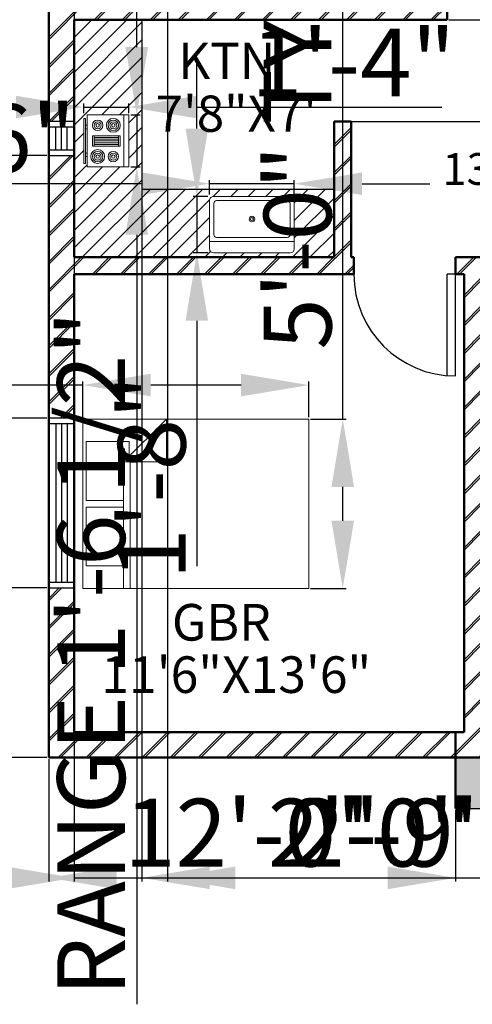
# Model space of a CAD drawing. Units: inches. Extents: x -584 to 444, y 228 to 1001.
# Tile 2 of 5: x -228 to -68, y 298 to 647. Entities that reach past the tile are written whole.
import ezdxf

# ---------------------------------------------------------------- set-up
doc = ezdxf.new("R2010")
doc.units = ezdxf.units.IN
for name, color, linetype, lineweight in [('A-ANNO-DIMS', 2, 'Continuous', 18), ('A-AREA-IDEN', 7, 'Continuous', 25), ('A-DOOR', 3, 'Continuous', 25), ('A-EQPM', 8, 'Continuous', 18), ('A-FLOR-CASE', 8, 'Continuous', 25), ('A-FLOR-CASE-PATT', 252, 'Continuous', 13), ('A-FLOR-FIXT', 9, 'Continuous', 18), ('A-FLOR-STRS', 7, 'Continuous', 25), ('A-FURN', 8, 'Continuous', 18), ('A-GLAZ', 4, 'Continuous', 25), ('A-WALL', 7, 'Continuous', 50), ('A-WALL-PATT', 3, 'Continuous', 13)]:
    doc.layers.add(name, color=color, linetype=linetype, lineweight=lineweight)
doc.styles.get("Standard").update_dxf_attribs({"font": 'arial.ttf'})
doc.dimstyles.new('ISO-25', dxfattribs={"dimtxt": 24, "dimasz": 24, "dimexe": 1.25, "dimexo": 0.625, "dimtad": 1, "dimdec": 1, "dimlunit": 3, "dimtxsty": 'Standard', "dimcen": 2.5, "dimadec": 0, "dimazin": 0, "dimtfac": 1, "dimtdec": 1, "dimtmove": 0, "dimatfit": 3, "dimfxl": 1, "dimarcsym": 0})

# ---------------------------------------------------------------- blocks, each defined once
blk = doc.blocks.new('Sink-single - 30 in top')
blk.add_line((-15, -3.999996), (15, -3.999996))
for points in [[(-13.5, 0), (13.5, 0)], [(-15, -18.499996), (-15, -1.5)], [(15, -1.5), (15, -18.499996)], [(-13.5, -17.499996), (-13.5, -6.499996)], [(-12.5, -5.499996), (12.5, -5.499996)], [(13.5, -6.499996), (13.5, -17.499996)], [(13.5, -19.999996), (-13.5, -19.999996)], [(12.5, -18.499996), (-12.5, -18.499996)]]:
    blk.add_lwpolyline(points)
for radius in [1, 0.5]:
    blk.add_circle((0, -11.999996), radius)
for centre, radius, start, end in [((-13.5, -1.5), 1.5, 90, 180), ((13.5, -1.5), 1.5, 0, 90), ((-12.5, -6.499996), 1, 90, 180), ((12.5, -6.499996), 1, 0, 90), ((-13.5, -18.499996), 1.5, 180, 270), ((-12.5, -17.499996), 1, 180, 270), ((12.5, -17.499996), 1, 270, 0), ((13.5, -18.499996), 1.5, 270, 0)]:
    blk.add_arc(centre, radius, start, end)
blk = doc.blocks.new('Range-Oven - 30 in top')
for p, q in [((0, -3), (30, -3)), ((12, -6), (18, -6)), ((13, -20), (13, -6)), ((14, -6), (14, -20)), ((15, -20), (15, -6)), ((16, -6), (16, -20)), ((17, -20), (17, -6)), ((18, -20), (12, -20)), ((6, -24), (6, -25)), ((8, -25), (8, -24)), ((22, -25), (22, -24)), ((24, -24), (24, -25))]:
    blk.add_line(p, q)
for points in [[(0, -24), (0, 0), (30, 0), (30, -24)], [(12, -21), (12, -5), (18, -5), (18, -21)], [(2, -26), (2, -25), (28, -25), (28, -26)]]:
    blk.add_lwpolyline(points, close=True)
for centre, radius in [((6, -9), 4), ((6, -9), 3), ((6, -9), 2), ((6, -9), 1), ((24, -9), 3), ((24, -9), 2), ((24, -9), 1), ((6, -18), 3), ((6, -18), 2), ((6, -18), 1), ((24, -18), 4), ((24, -18), 3), ((24, -18), 2), ((24, -18), 1)]:
    blk.add_circle(centre, radius)
blk = doc.blocks.new('Bed - Queen')
for p, q in [((0, -80.00003), (0, 0)), ((0, 0), (59.99999, 0)), ((59.99999, 0), (59.99999, -80.00003)), ((7.99999, -1.2), (28.79998, -1.2)), ((7.99999, -14.4), (7.99999, -1.2)), ((28.79998, -1.2), (28.79998, -14.4)), ((31.19999, -1.2), (51.99999, -1.2)), ((31.19999, -14.4), (31.19999, -1.2)), ((51.99999, -1.2), (51.99999, -16.4)), ((0, -14.4), (44.8, -14.4)), ((44.8, -16.8), (0, -16.8)), ((59.99999, -29.6), (44.8, -14.4)), ((44.8, -14.4), (44.8, -29.6)), ((51.99999, -16.4), (46.79936, -16.4)), ((44.8, -29.6), (59.99999, -29.6)), ((59.99999, -80.00003), (0, -80.00003))]:
    blk.add_line(p, q)
blk = doc.blocks.new('WIN-60IN')
for p, q in [((60, 9), (0, 9)), ((0, 9), (0, 0)), ((2, 9), (2, 0)), ((58, 0), (58, 9)), ((60, 0), (60, 9)), ((2, 6.5), (58, 6.5)), ((2, 4.5), (58, 4.5)), ((0, 0), (60, 0)), ((2, 2.5), (58, 2.5))]:
    blk.add_line(p, q)
blk = doc.blocks.new('WIN-12IN')
for p, q in [((12, 9), (0, 9)), ((0, 9), (0, 0)), ((2, 9), (2, 0)), ((10, 0), (10, 9)), ((12, 0), (12, 9)), ((2, 6.5), (10, 6.5)), ((2, 4.5), (10, 4.5)), ((0, 0), (12, 0)), ((2, 2.5), (10, 2.5))]:
    blk.add_line(p, q)
blk = doc.blocks.new('DOOR-SWING-36IN')
for p, q in [((0, 36), (0, 0)), ((3, 36), (3, 0)), ((0, 0), (3, 0))]:
    blk.add_line(p, q)
blk.add_arc((0, 0), 36, 0, 90)
blk = doc.blocks.new('*D15')
at = {"layer": 'A-ANNO-DIMS', "color": 0, "lineweight": -2, "transparency": 16777216}
for p, q in [((-206.06, 517.3), (-584.35, 517.3)), ((-206.06, 505.93), (-206.06, 518.55)), ((-150.06, 517.3), (-182.06, 517.3)), ((-126.06, 505.93), (-126.06, 518.55))]:
    blk.add_line(p, q, dxfattribs=at)
at = {"layer": 'A-ANNO-DIMS', "color": 0, "transparency": 16777216}
for points in [[(-182.06, 521.3), (-182.06, 513.3), (-206.06, 517.3)], [(-150.06, 521.3), (-150.06, 513.3), (-126.06, 517.3)]]:
    blk.add_solid(points, dxfattribs=at)
at = {"layer": 'Defpoints', "color": 0, "transparency": 16777216}
for p in [(-206.06, 517.3), (-206.06, 505.3), (-126.06, 505.3)]:
    blk.add_point(p, dxfattribs=at)
at = {"layer": 'A-ANNO-DIMS', "color": 0, "transparency": 16777216, "insert": (-407.21, 531.07), "char_height": 24, "attachment_point": 5}
blk.add_mtext('QUEEN BED 6\'-8" TYP.', dxfattribs=at)
blk = doc.blocks.new('*D16')
at = {"layer": 'A-ANNO-DIMS', "color": 0, "lineweight": -2, "transparency": 16777216}
for p, q in [((-114.06, 505.3), (-114.06, 676.85)), ((-125.44, 505.3), (-112.81, 505.3)), ((-114.06, 469.3), (-114.06, 481.3)), ((-125.44, 445.3), (-112.81, 445.3))]:
    blk.add_line(p, q, dxfattribs=at)
at = {"layer": 'A-ANNO-DIMS', "color": 0, "transparency": 16777216}
for points in [[(-118.06, 481.3), (-110.06, 481.3), (-114.06, 505.3)], [(-118.06, 469.3), (-110.06, 469.3), (-114.06, 445.3)]]:
    blk.add_solid(points, dxfattribs=at)
at = {"layer": 'Defpoints', "color": 0, "transparency": 16777216}
for p in [(-126.06, 505.3), (-114.06, 505.3), (-126.06, 445.3)]:
    blk.add_point(p, dxfattribs=at)
at = {"layer": 'A-ANNO-DIMS', "color": 0, "transparency": 16777216, "insert": (-126.94, 603.07), "char_height": 24, "attachment_point": 5, "rotation": 90}
blk.add_mtext('5\'-0" TYP.', dxfattribs=at)
blk = doc.blocks.new('*D19')
at = {"layer": 'A-ANNO-DIMS', "color": 0, "lineweight": -2, "transparency": 16777216}
for p, q in [((-161.21, 584.69), (-161.21, 589.81)), ((-131.21, 584.69), (-131.21, 589.81)), ((-185.21, 588.56), (-361.72, 588.56)), ((-131.21, 588.56), (-161.21, 588.56)), ((-107.21, 588.56), (-83.21, 588.56))]:
    blk.add_line(p, q, dxfattribs=at)
at = {"layer": 'A-ANNO-DIMS', "color": 0, "transparency": 16777216}
for points in [[(-185.21, 592.56), (-185.21, 584.56), (-161.21, 588.56)], [(-107.21, 592.56), (-107.21, 584.56), (-131.21, 588.56)]]:
    blk.add_solid(points, dxfattribs=at)
at = {"layer": 'Defpoints', "color": 0, "transparency": 16777216}
for p in [(-161.21, 588.56), (-161.21, 584.06), (-131.21, 584.06)]:
    blk.add_point(p, dxfattribs=at)
at = {"layer": 'A-ANNO-DIMS', "color": 0, "transparency": 16777216, "insert": (-285.47, 601.6), "char_height": 24, "attachment_point": 5}
blk.add_mtext('SINK 2\'-6"', dxfattribs=at)
blk = doc.blocks.new('*D20')
at = {"layer": 'A-ANNO-DIMS', "color": 0, "lineweight": -2, "transparency": 16777216}
for p, q in [((-165.71, 608.06), (-165.71, 632.06)), ((-161.84, 584.06), (-166.96, 584.06)), ((-165.71, 584.06), (-165.71, 564.06)), ((-161.84, 564.06), (-166.96, 564.06)), ((-165.71, 540.06), (-165.71, 453.27))]:
    blk.add_line(p, q, dxfattribs=at)
at = {"layer": 'A-ANNO-DIMS', "color": 0, "transparency": 16777216}
for points in [[(-169.71, 608.06), (-161.71, 608.06), (-165.71, 584.06)], [(-169.71, 540.06), (-161.71, 540.06), (-165.71, 564.06)]]:
    blk.add_solid(points, dxfattribs=at)
at = {"layer": 'Defpoints', "color": 0, "transparency": 16777216}
for p in [(-161.21, 584.06), (-165.71, 564.06), (-161.21, 564.06)]:
    blk.add_point(p, dxfattribs=at)
at = {"layer": 'A-ANNO-DIMS', "color": 0, "transparency": 16777216, "insert": (-178.59, 484.67), "char_height": 24, "attachment_point": 5, "rotation": 90}
blk.add_mtext('1\'-8"', dxfattribs=at)
blk = doc.blocks.new('*D21')
at = {"layer": 'A-ANNO-DIMS', "color": 0, "lineweight": -2, "transparency": 16777216}
for p, q in [((-186.99, 636.91), (-186.99, 660.91)), ((-189.13, 612.91), (-185.74, 612.91)), ((-186.99, 612.91), (-186.99, 594.47)), ((-189.13, 594.47), (-185.74, 594.47)), ((-186.99, 570.47), (-186.99, 298.2))]:
    blk.add_line(p, q, dxfattribs=at)
at = {"layer": 'A-ANNO-DIMS', "color": 0, "transparency": 16777216}
for points in [[(-190.99, 636.91), (-182.99, 636.91), (-186.99, 612.91)], [(-190.99, 570.47), (-182.99, 570.47), (-186.99, 594.47)]]:
    blk.add_solid(points, dxfattribs=at)
at = {"layer": 'Defpoints', "color": 0, "transparency": 16777216}
for p in [(-189.76, 612.91), (-189.76, 594.47), (-186.99, 594.47)]:
    blk.add_point(p, dxfattribs=at)
at = {"layer": 'A-ANNO-DIMS', "color": 0, "transparency": 16777216, "insert": (-200.02, 422.34), "char_height": 24, "attachment_point": 5, "rotation": 90}
blk.add_mtext('RANGE 1\'-6 1/2"', dxfattribs=at)
blk = doc.blocks.new('*D22')
at = {"layer": 'A-ANNO-DIMS', "color": 0, "lineweight": -2, "transparency": 16777216}
for p, q in [((-205.74, 613.54), (-205.74, 616.93)), ((-189.76, 613.54), (-189.76, 616.93)), ((-229.74, 615.68), (-253.74, 615.68)), ((-205.74, 615.68), (-189.76, 615.68)), ((-165.76, 615.68), (-78.97, 615.68))]:
    blk.add_line(p, q, dxfattribs=at)
at = {"layer": 'A-ANNO-DIMS', "color": 0, "transparency": 16777216}
for points in [[(-229.74, 619.68), (-229.74, 611.68), (-205.74, 615.68)], [(-165.76, 619.68), (-165.76, 611.68), (-189.76, 615.68)]]:
    blk.add_solid(points, dxfattribs=at)
at = {"layer": 'Defpoints', "color": 0, "transparency": 16777216}
for p in [(-189.76, 615.68), (-205.74, 612.91), (-189.76, 612.91)]:
    blk.add_point(p, dxfattribs=at)
at = {"layer": 'A-ANNO-DIMS', "color": 0, "transparency": 16777216, "insert": (-110.36, 628.35), "char_height": 24, "attachment_point": 5}
blk.add_mtext('1\'-4"', dxfattribs=at)
blk = doc.blocks.new('*D28')
at = {"layer": 'A-ANNO-DIMS', "color": 0, "lineweight": -2, "transparency": 16777216}
for p, q in [((-218.14, 384.91), (-218.14, 341.69)), ((-74.14, 366.91), (-74.14, 341.69)), ((-194.14, 342.94), (-98.14, 342.94))]:
    blk.add_line(p, q, dxfattribs=at)
at = {"layer": 'A-ANNO-DIMS', "color": 0, "transparency": 16777216}
for points in [[(-194.14, 346.94), (-194.14, 338.94), (-218.14, 342.94)], [(-98.14, 346.94), (-98.14, 338.94), (-74.14, 342.94)]]:
    blk.add_solid(points, dxfattribs=at)
at = {"layer": 'Defpoints', "color": 0, "transparency": 16777216}
for p in [(-218.14, 385.54), (-74.14, 367.54), (-74.14, 342.94)]:
    blk.add_point(p, dxfattribs=at)
at = {"layer": 'A-ANNO-DIMS', "color": 0, "transparency": 16777216, "insert": (-146.14, 355.82), "char_height": 24, "attachment_point": 5}
blk.add_mtext('12\'-0"', dxfattribs=at)
blk = doc.blocks.new('*D29')
at = {"layer": 'A-ANNO-DIMS', "color": 0, "lineweight": -2, "transparency": 16777216}
for p, q in [((-209.14, 795.91), (-209.14, 341.69)), ((-176.14, 795.91), (-176.14, 341.69)), ((-233.14, 342.94), (-257.14, 342.94)), ((-209.14, 342.94), (-176.14, 342.94)), ((-152.14, 342.94), (-62.69, 342.94))]:
    blk.add_line(p, q, dxfattribs=at)
at = {"layer": 'A-ANNO-DIMS', "color": 0, "transparency": 16777216}
for points in [[(-233.14, 346.94), (-233.14, 338.94), (-209.14, 342.94)], [(-152.14, 346.94), (-152.14, 338.94), (-176.14, 342.94)]]:
    blk.add_solid(points, dxfattribs=at)
at = {"layer": 'Defpoints', "color": 0, "transparency": 16777216}
for p in [(-209.14, 796.54), (-176.14, 796.54), (-176.14, 342.94)]:
    blk.add_point(p, dxfattribs=at)
at = {"layer": 'A-ANNO-DIMS', "color": 0, "transparency": 16777216, "insert": (-95.41, 355.82), "char_height": 24, "attachment_point": 5}
blk.add_mtext('2\'-9"', dxfattribs=at)
blk = doc.blocks.new('*D33')
at = {"layer": 'A-ANNO-DIMS', "color": 0, "lineweight": -2, "transparency": 16777216}
for p, q in [((-242.74, 445.54), (-242.74, 534.59)), ((-218.77, 445.54), (-243.99, 445.54)), ((-242.74, 409.54), (-242.74, 421.54)), ((-218.77, 385.54), (-243.99, 385.54))]:
    blk.add_line(p, q, dxfattribs=at)
at = {"layer": 'A-ANNO-DIMS', "color": 0, "transparency": 16777216}
for points in [[(-246.74, 421.54), (-238.74, 421.54), (-242.74, 445.54)], [(-246.74, 409.54), (-238.74, 409.54), (-242.74, 385.54)]]:
    blk.add_solid(points, dxfattribs=at)
at = {"layer": 'Defpoints', "color": 0, "transparency": 16777216}
for p in [(-242.74, 445.54), (-218.14, 445.54), (-218.14, 385.54)]:
    blk.add_point(p, dxfattribs=at)
at = {"layer": 'A-ANNO-DIMS', "color": 0, "transparency": 16777216, "insert": (-255.62, 502.06), "char_height": 24, "attachment_point": 5, "rotation": 90}
blk.add_mtext('5\'-0"', dxfattribs=at)
blk = doc.blocks.new('*D34')
at = {"layer": 'A-ANNO-DIMS', "color": 0, "lineweight": -2, "transparency": 16777216}
for p, q in [((-218.77, 598.54), (-243.99, 598.54)), ((-242.74, 529.54), (-242.74, 574.54)), ((-218.77, 505.54), (-243.99, 505.54))]:
    blk.add_line(p, q, dxfattribs=at)
at = {"layer": 'A-ANNO-DIMS', "color": 0, "transparency": 16777216}
for points in [[(-246.74, 574.54), (-238.74, 574.54), (-242.74, 598.54)], [(-246.74, 529.54), (-238.74, 529.54), (-242.74, 505.54)]]:
    blk.add_solid(points, dxfattribs=at)
at = {"layer": 'Defpoints', "color": 0, "transparency": 16777216}
for p in [(-242.74, 598.54), (-218.14, 598.54), (-218.14, 505.54)]:
    blk.add_point(p, dxfattribs=at)
at = {"layer": 'A-ANNO-DIMS', "color": 0, "transparency": 16777216, "insert": (-255.62, 552.04), "char_height": 24, "attachment_point": 5, "rotation": 90}
blk.add_mtext('7\'-9"', dxfattribs=at)
blk = doc.blocks.new('*D39')
at = {"layer": 'A-ANNO-DIMS', "color": 0, "lineweight": -2, "transparency": 16777216}
for p, q in [((-209.14, 645.91), (-209.14, 341.69)), ((-185.14, 645.91), (-185.14, 341.69)), ((-233.14, 342.94), (-257.14, 342.94)), ((-209.14, 342.94), (-185.14, 342.94)), ((-161.14, 342.94), (-71.69, 342.94))]:
    blk.add_line(p, q, dxfattribs=at)
at = {"layer": 'A-ANNO-DIMS', "color": 0, "transparency": 16777216}
for points in [[(-233.14, 346.94), (-233.14, 338.94), (-209.14, 342.94)], [(-161.14, 346.94), (-161.14, 338.94), (-185.14, 342.94)]]:
    blk.add_solid(points, dxfattribs=at)
at = {"layer": 'Defpoints', "color": 0, "transparency": 16777216}
for p in [(-209.14, 646.54), (-185.14, 646.54), (-185.14, 342.94)]:
    blk.add_point(p, dxfattribs=at)
at = {"layer": 'A-ANNO-DIMS', "color": 0, "transparency": 16777216, "insert": (-104.41, 355.82), "char_height": 24, "attachment_point": 5}
blk.add_mtext('2\'-0"', dxfattribs=at)
blk = doc.blocks.new('*D40')
at = {"layer": 'A-ANNO-DIMS', "color": 0, "lineweight": -2, "transparency": 16777216}
for p, q in [((130.46, 670.54), (130.46, 759.57)), ((-76.52, 646.54), (131.71, 646.54)), ((130.46, 610.54), (130.46, 646.54)), ((-116.52, 610.54), (131.71, 610.54)), ((130.46, 586.54), (130.46, 562.54))]:
    blk.add_line(p, q, dxfattribs=at)
at = {"layer": 'A-ANNO-DIMS', "color": 0, "transparency": 16777216}
for points in [[(126.46, 670.54), (134.46, 670.54), (130.46, 646.54)], [(126.46, 586.54), (134.46, 586.54), (130.46, 610.54)]]:
    blk.add_solid(points, dxfattribs=at)
at = {"layer": 'Defpoints', "color": 0, "transparency": 16777216}
for p in [(-77.14, 646.54), (130.46, 646.54), (-117.14, 610.54)]:
    blk.add_point(p, dxfattribs=at)
at = {"layer": 'A-ANNO-DIMS', "color": 0, "transparency": 16777216, "insert": (117.57, 727.05), "char_height": 24, "attachment_point": 5, "rotation": 90}
blk.add_mtext('3\'-0"', dxfattribs=at)
blk = doc.blocks.new('*D41')
at = {"layer": 'A-ANNO-DIMS', "color": 0, "lineweight": -2, "transparency": 16777216}
for p, q in [((-89.14, 830.14), (-113.14, 830.14)), ((-65.14, 563.16), (-65.14, 831.39)), ((-65.14, 830.14), (-29.14, 830.14)), ((-29.14, 528.16), (-29.14, 831.39)), ((-5.14, 830.14), (83.89, 830.14))]:
    blk.add_line(p, q, dxfattribs=at)
at = {"layer": 'A-ANNO-DIMS', "color": 0, "transparency": 16777216}
for points in [[(-89.14, 834.14), (-89.14, 826.14), (-65.14, 830.14)], [(-5.14, 834.14), (-5.14, 826.14), (-29.14, 830.14)]]:
    blk.add_solid(points, dxfattribs=at)
at = {"layer": 'Defpoints', "color": 0, "transparency": 16777216}
for p in [(-29.14, 830.14), (-65.14, 562.54), (-29.14, 527.54)]:
    blk.add_point(p, dxfattribs=at)
at = {"layer": 'A-ANNO-DIMS', "color": 0, "transparency": 16777216, "insert": (51.37, 843.02), "char_height": 24, "attachment_point": 5}
blk.add_mtext('3\'-0"', dxfattribs=at)

msp = doc.modelspace()

# ---------------------------------------------------------------- hatches: boundary and pattern name
at = {"layer": 'A-FLOR-CASE-PATT'}
h = msp.add_hatch(dxfattribs=at)
h.set_pattern_fill('JIS_WOOD', color=256, scale=6.2)
h.paths.add_polyline_path([(-117.14, 586.54), (-185.14, 586.54), (-185.14, 646.54), (-209.14, 646.54), (-209.14, 562.54), (-117.14, 562.54)])
h.paths.add_polyline_path([(-204.51, 594.47), (-204.51, 598.16), (-205.12, 598.16), (-205.12, 595.7), (-205.74, 595.7), (-205.74, 611.68), (-205.12, 611.68), (-205.12, 609.23), (-204.51, 609.23), (-204.51, 612.91), (-189.76, 612.91), (-189.76, 594.47)], flags=16)
h.paths.add_polyline_path([(-197.13, 598.16, -1), (-193.44, 598.16, -1)], flags=0)
h.paths.add_polyline_path([(-203.28, 598.16, -1), (-198.36, 598.16, -1)], flags=0)
h.paths.add_polyline_path([(-196.52, 598.16, -1), (-194.06, 598.16, -1)], flags=0)
h.paths.add_polyline_path([(-202.66, 598.16, -1), (-198.98, 598.16, -1)], flags=0)
h.paths.add_polyline_path([(-195.9, 598.16, -1), (-194.67, 598.16, -1)], flags=0)
h.paths.add_polyline_path([(-202.05, 598.16, -1), (-199.59, 598.16, -1)], flags=0)
h.paths.add_polyline_path([(-201.43, 598.16, -1), (-200.2, 598.16, -1)], flags=0)
h.paths.add_polyline_path([(-202.66, 601.85), (-202.66, 605.54), (-192.83, 605.54), (-192.83, 601.85)], flags=0)
h.paths.add_polyline_path([(-193.44, 602.46), (-202.05, 602.46), (-202.05, 604.92), (-193.44, 604.92)], flags=0)
h.paths.add_polyline_path([(-197.75, 609.23, -1), (-192.83, 609.23, -1)], flags=0)
h.paths.add_polyline_path([(-197.13, 609.23, -1), (-193.44, 609.23, -1)], flags=0)
h.paths.add_polyline_path([(-196.52, 609.23, -1), (-194.06, 609.23, -1)], flags=0)
h.paths.add_polyline_path([(-202.66, 609.23, -1), (-198.98, 609.23, -1)], flags=0)
h.paths.add_polyline_path([(-195.9, 609.23, -1), (-194.67, 609.23, -1)], flags=0)
h.paths.add_polyline_path([(-202.05, 609.23, -1), (-199.59, 609.23, -1)], flags=0)
h.paths.add_polyline_path([(-201.43, 609.23, -1), (-200.2, 609.23, -1)], flags=0)
h.paths.add_polyline_path([(-161.21, 582.56, -0.414214), (-159.71, 584.06), (-132.71, 584.06, -0.414214), (-131.21, 582.56), (-131.21, 565.56, -0.414214), (-132.71, 564.06), (-159.71, 564.06, -0.414214), (-161.21, 565.56)], flags=16)
h.paths.add_polyline_path([(-159.71, 581.56, -0.414214), (-158.71, 582.56), (-133.71, 582.56, -0.414214), (-132.71, 581.56), (-132.71, 570.56, -0.414214), (-133.71, 569.56), (-158.71, 569.56, -0.414214), (-159.71, 570.56)], flags=0)
h.paths.add_polyline_path([(-145.21, 576.06, -1), (-147.21, 576.06, -1)], flags=0)
h.paths.add_polyline_path([(-145.71, 576.06, -1), (-146.71, 576.06, -1)], flags=0)
at = {"layer": 'A-WALL-PATT'}
h = msp.add_hatch(dxfattribs=at)
h.set_pattern_fill('JIS_LC_8A', color=256, scale=0.9)
h.set_pattern_definition([(45, (105.857, 805.537), (-4.96389, 4.96389), []), (45, (106.757, 805.537), (-4.96389, 4.96389), [])])
h.paths.add_polyline_path([(105.86, 694.54), (96.86, 694.54), (96.86, 652.54), (15.86, 652.54), (15.86, 646.54), (96.86, 646.54), (96.86, 617.04), (105.86, 617.04)])
h.paths.add_polyline_path([(-77.14, 655.54), (-83.14, 655.54), (-83.14, 652.54), (-209.14, 652.54), (-209.14, 796.54), (-176.14, 796.54), (-176.14, 805.54), (-218.14, 805.54), (-218.14, 610.54), (-209.14, 610.54), (-209.14, 646.54), (-77.14, 646.54)])
h.paths.add_polyline_path([(-209.14, 598.54), (-218.14, 598.54), (-218.14, 505.54), (-209.14, 505.54), (-209.14, 556.54), (-111.14, 556.54), (-110.14, 556.54), (-110.14, 562.54), (-111.14, 562.54), (-111.14, 610.54), (-117.14, 610.54), (-117.14, 562.54), (-209.14, 562.54)])
h.paths.add_polyline_path([(-59.14, 805.54), (-116.14, 805.54), (-116.14, 796.54), (-83.14, 796.54), (-83.14, 691.54), (-77.14, 691.54), (-77.14, 796.54), (-59.14, 796.54)])
h.paths.add_polyline_path([(105.86, 805.54), (-47.14, 805.54), (-47.14, 796.54), (-29.14, 796.54), (-29.14, 712.54), (-47.14, 712.54), (-47.14, 706.54), (-29.14, 706.54), (-29.14, 646.54), (-20.14, 646.54), (-20.14, 652.54), (-23.14, 652.54), (-23.14, 796.54), (96.86, 796.54), (96.86, 754.54), (105.86, 754.54)])
h.paths.add_polyline_path([(-65.14, 385.54), (-65.14, 562.54), (-71.14, 562.54), (-74.14, 562.54), (-74.14, 556.54), (-71.14, 556.54), (-71.14, 394.54), (-209.14, 394.54), (-209.14, 445.54), (-218.14, 445.54), (-218.14, 385.54)])
h = msp.add_hatch(dxfattribs=at)
h.set_pattern_fill('BRICK', color=256, scale=0.2)
h.paths.add_polyline_path([(-65.14, 385.54), (-74.14, 385.54), (-74.14, 367.54), (-65.14, 367.54)])
h.paths.add_polyline_path([(105.86, 385.54), (96.86, 385.54), (96.86, 367.54), (105.86, 367.54)])

# ---------------------------------------------------------------- linework, layer by layer
at = {"layer": 'A-FLOR-CASE'}
for p in [(-185.14, 646.54), (-117.14, 586.54)]:
    msp.add_line(p, (-185.14, 586.54), dxfattribs=at)
at = {"layer": 'A-FLOR-STRS'}
msp.add_line((-74.14, 367.54), (105.86, 367.54), dxfattribs=at)
at = {"layer": 'A-WALL'}
for p, q in [((-218.14, 805.54), (-218.14, 385.54)), ((-77.14, 655.54), (-77.14, 646.54)), ((-77.14, 646.54), (-209.14, 646.54)), ((-209.14, 646.54), (-209.14, 562.54)), ((-111.14, 610.54), (-117.14, 610.54)), ((-117.14, 610.54), (-117.14, 562.54)), ((-111.14, 610.54), (-111.14, 562.54)), ((-117.14, 562.54), (-209.14, 562.54)), ((-110.14, 562.54), (-111.14, 562.54)), ((-110.14, 556.54), (-110.14, 562.54)), ((-74.14, 556.54), (-74.14, 562.54)), ((-71.14, 562.54), (-74.14, 562.54)), ((-71.14, 562.54), (-65.14, 562.54)), ((-111.14, 556.54), (-209.14, 556.54)), ((-209.14, 556.54), (-111.14, 556.54)), ((-209.14, 556.54), (-209.14, 394.54)), ((-110.14, 556.54), (-111.14, 556.54)), ((-71.14, 556.54), (-74.14, 556.54)), ((-71.14, 556.54), (-71.14, 394.54)), ((-209.14, 394.54), (-71.14, 394.54)), ((-74.14, 394.54), (-74.14, 367.54)), ((-218.14, 385.54), (105.86, 385.54))]:
    msp.add_line(p, q, dxfattribs=at)

# ---------------------------------------------------------------- block references
at = {"layer": 'A-DOOR', "rotation": 180}
msp.add_blockref('DOOR-SWING-36IN', (-74.14, 556.54), dxfattribs=at)
at = {"layer": 'A-EQPM', "xscale": 0.6146363072762816, "yscale": 0.6146363072762816, "zscale": 0.6146363072762816, "rotation": 270}
msp.add_blockref('Range-Oven - 30 in top', (-189.76, 612.91), dxfattribs=at)
at = {"layer": 'A-FLOR-FIXT', "rotation": 180}
msp.add_blockref('Sink-single - 30 in top', (-146.21, 564.06), dxfattribs=at)
at = {"layer": 'A-FURN', "rotation": 90}
msp.add_blockref('Bed - Queen', (-206.06, 445.3), dxfattribs=at)
at = {"layer": 'A-GLAZ'}
for name, p, rotation in [('WIN-12IN', (-209.14, 598.54), 89.99999999999916), ('WIN-60IN', (-218.14, 505.54), 270.0000000000002)]:
    msp.add_blockref(name, p, dxfattribs=dict(at, rotation=rotation))

# ---------------------------------------------------------------- texts
at = {"layer": 'A-AREA-IDEN', "attachment_point": 1}
for s, width, gutter_width, insert, char_height in [('KTN', 740.4842, 64.06, (-172.28, 638.46), 12.812), ('7\'8"X7\'', 740.4842, 64.06, (-180.3, 619.74), 12.812), ('13\'6"X9\'11"', 648.8713, 56.13, (-78.72, 599.38), 11.2267), ('GBR', 748.4344, 64.75, (-174.52, 439.85), 12.949), ('11\'6"X13\'6"', 748.4344, 64.75, (-199.52, 421.33), 12.9493)]:
    msp.add_mtext_dynamic_manual_height_columns(s, width=width, gutter_width=gutter_width, heights=[0], dxfattribs=dict(at, insert=insert, char_height=char_height))

# ---------------------------------------------------------------- dimensions: what is measured, and where the dimension line sits
at = {"layer": 'A-ANNO-DIMS'}
for base, p1, p2, picture, middle in [((-29.14, 830.14), (-65.14, 562.54), (-29.14, 527.54), '*D41', (51.37, 843.02)), ((-176.14, 342.94), (-209.14, 796.54), (-176.14, 796.54), '*D29', (-95.41, 355.82)), ((-185.14, 342.94), (-209.14, 646.54), (-185.14, 646.54), '*D39', (-104.41, 355.82)), ((-189.76, 615.68), (-205.74, 612.91), (-189.76, 612.91), '*D22', (-110.36, 628.35)), ((-74.14, 342.94), (-218.14, 385.54), (-74.14, 367.54), '*D28', (-146.14, 355.82))]:
    dim = msp.add_linear_dim(base=base, p1=p1, p2=p2, dimstyle='ISO-25', override={"dimdec": 1, "dimlfac": 1, "dimrnd": 0, "dimzin": 1, "dimdsep": 46, "dimlunit": 4, "dimfrac": 2}, dxfattribs=at)
    dim.commit()
    dim.dimension.update_dxf_attribs({"geometry": picture, "text_midpoint": middle})
for base, p1, p2, angle, picture, middle in [((130.46, 646.54), (-117.14, 610.54), (-77.14, 646.54), 90, '*D40', (117.57, 727.05)), ((-165.71, 564.06), (-161.21, 584.06), (-161.21, 564.06), 270, '*D20', (-178.59, 484.67)), ((-242.74, 598.54), (-218.14, 505.54), (-218.14, 598.54), 90, '*D34', (-255.62, 552.04)), ((-242.74, 445.54), (-218.14, 385.54), (-218.14, 445.54), 90, '*D33', (-255.62, 502.06))]:
    dim = msp.add_linear_dim(base=base, p1=p1, p2=p2, angle=angle, dimstyle='ISO-25', override={"dimdec": 1, "dimlfac": 1, "dimrnd": 0, "dimzin": 1, "dimdsep": 46, "dimlunit": 4, "dimfrac": 2}, dxfattribs=at)
    dim.commit()
    dim.dimension.update_dxf_attribs({"geometry": picture, "text_midpoint": middle})
for base, p1, p2, angle, text, picture, middle in [((-114.06, 505.3), (-126.06, 445.3), (-126.06, 505.3), 90, '<> TYP.', '*D16', (-126.94, 603.07)), ((-186.99, 594.47), (-189.76, 612.91), (-189.76, 594.47), 270, 'RANGE <>', '*D21', (-200.02, 422.34)), ((-161.21, 588.56), (-131.21, 584.06), (-161.21, 584.06), 180, 'SINK <>', '*D19', (-285.47, 601.6)), ((-206.06, 517.3), (-126.06, 505.3), (-206.06, 505.3), 180, 'QUEEN BED <> TYP.', '*D15', (-407.21, 531.07))]:
    dim = msp.add_linear_dim(base=base, p1=p1, p2=p2, angle=angle, text=text, dimstyle='ISO-25', override={"dimdec": 1, "dimlfac": 1, "dimrnd": 0, "dimzin": 1, "dimdsep": 46, "dimlunit": 4, "dimfrac": 2}, dxfattribs=at)
    dim.commit()
    dim.dimension.update_dxf_attribs({"geometry": picture, "text_midpoint": middle})

doc.saveas('drawing.dxf')
